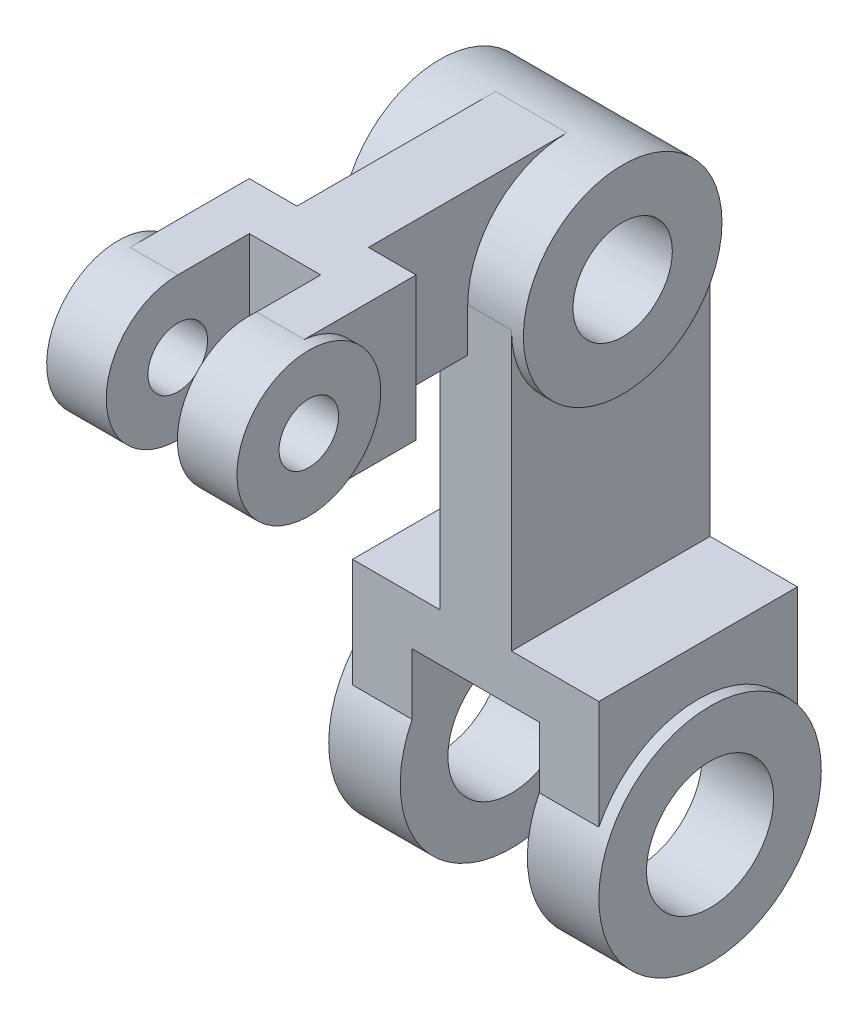
ISO-10303-21;
HEADER;
FILE_DESCRIPTION(('STEP AP214'),'2;1');
FILE_NAME('part.step','',(''),(''),'','','');
FILE_SCHEMA(('AUTOMOTIVE_DESIGN { 1 0 10303 214 1 1 1 1 }'));
ENDSEC;
DATA;
#1=APPLICATION_CONTEXT('core data for automotive mechanical design processes');
#2=APPLICATION_PROTOCOL_DEFINITION('international standard','automotive_design',2000,#1);
#3=PRODUCT_CONTEXT('',#1,'mechanical');
#4=PRODUCT('Part','Part','',(#3));
#5=PRODUCT_RELATED_PRODUCT_CATEGORY('part','',(#4));
#6=PRODUCT_DEFINITION_FORMATION('','',#4);
#7=PRODUCT_DEFINITION_CONTEXT('part definition',#1,'design');
#8=PRODUCT_DEFINITION('design','',#6,#7);
#9=PRODUCT_DEFINITION_SHAPE('','',#8);
#10=(LENGTH_UNIT() NAMED_UNIT(*) SI_UNIT(.MILLI.,.METRE.));
#11=(NAMED_UNIT(*) PLANE_ANGLE_UNIT() SI_UNIT($,.RADIAN.));
#12=(NAMED_UNIT(*) SI_UNIT($,.STERADIAN.) SOLID_ANGLE_UNIT());
#13=UNCERTAINTY_MEASURE_WITH_UNIT(LENGTH_MEASURE(1.E-05),#10,'distance_accuracy_value','');
#14=(GEOMETRIC_REPRESENTATION_CONTEXT(3) GLOBAL_UNCERTAINTY_ASSIGNED_CONTEXT((#13)) GLOBAL_UNIT_ASSIGNED_CONTEXT((#10,
#11,#12)) REPRESENTATION_CONTEXT('',''));
#15=CARTESIAN_POINT('',(0.,0.,0.));
#16=DIRECTION('',(0.,0.,1.));
#17=DIRECTION('',(1.,0.,0.));
#18=AXIS2_PLACEMENT_3D('',#15,#16,#17);
#19=CARTESIAN_POINT('',(-20.,71.,0.));
#20=DIRECTION('',(0.,-1.,0.));
#21=DIRECTION('',(0.,0.,-1.));
#22=AXIS2_PLACEMENT_3D('',#19,#20,#21);
#23=PLANE('',#22);
#24=DIRECTION('',(0.,0.,-1.));
#25=VECTOR('',#24,1.);
#26=CARTESIAN_POINT('',(9.99999999999999,71.,80.));
#27=LINE('',#26,#25);
#28=CARTESIAN_POINT('',(9.99999999999999,71.,78.13652597627));
#29=VERTEX_POINT('',#28);
#30=CARTESIAN_POINT('',(9.99999999999999,71.,50.));
#31=VERTEX_POINT('',#30);
#32=EDGE_CURVE('E226',#29,#31,#27,.T.);
#33=ORIENTED_EDGE('',*,*,#32,.F.);
#34=DIRECTION('',(-1.,0.,0.));
#35=VECTOR('',#34,1.);
#36=CARTESIAN_POINT('',(13.,71.,78.13652597627));
#37=LINE('',#36,#35);
#38=CARTESIAN_POINT('',(-2.00000000000001,71.,78.13652597627));
#39=VERTEX_POINT('',#38);
#40=EDGE_CURVE('E520',#29,#39,#37,.T.);
#41=ORIENTED_EDGE('',*,*,#40,.T.);
#42=DIRECTION('',(0.,0.,1.));
#43=VECTOR('',#42,1.);
#44=CARTESIAN_POINT('',(-2.00000000000001,71.,62.));
#45=LINE('',#44,#43);
#46=CARTESIAN_POINT('',(-2.00000000000001,71.,62.));
#47=VERTEX_POINT('',#46);
#48=EDGE_CURVE('E246',#47,#39,#45,.T.);
#49=ORIENTED_EDGE('',*,*,#48,.F.);
#50=DIRECTION('',(1.,0.,0.));
#51=VECTOR('',#50,1.);
#52=CARTESIAN_POINT('',(-2.00000000000001,71.,62.));
#53=LINE('',#52,#51);
#54=CARTESIAN_POINT('',(-20.,71.,62.));
#55=VERTEX_POINT('',#54);
#56=EDGE_CURVE('E244',#55,#47,#53,.T.);
#57=ORIENTED_EDGE('',*,*,#56,.F.);
#58=DIRECTION('',(0.,0.,1.));
#59=VECTOR('',#58,1.);
#60=CARTESIAN_POINT('',(-20.,71.,62.));
#61=LINE('',#60,#59);
#62=CARTESIAN_POINT('',(-20.,71.,80.));
#63=VERTEX_POINT('',#62);
#64=EDGE_CURVE('E234',#55,#63,#61,.T.);
#65=ORIENTED_EDGE('',*,*,#64,.T.);
#66=DIRECTION('',(1.,0.,0.));
#67=VECTOR('',#66,1.);
#68=CARTESIAN_POINT('',(-32.,71.,80.));
#69=LINE('',#68,#67);
#70=CARTESIAN_POINT('',(-32.,71.,80.));
#71=VERTEX_POINT('',#70);
#72=EDGE_CURVE('E218',#71,#63,#69,.T.);
#73=ORIENTED_EDGE('',*,*,#72,.F.);
#74=DIRECTION('',(0.,0.,-1.));
#75=VECTOR('',#74,1.);
#76=CARTESIAN_POINT('',(-32.,71.,80.));
#77=LINE('',#76,#75);
#78=CARTESIAN_POINT('',(-32.,71.,50.));
#79=VERTEX_POINT('',#78);
#80=EDGE_CURVE('E272',#71,#79,#77,.T.);
#81=ORIENTED_EDGE('',*,*,#80,.T.);
#82=DIRECTION('',(1.,0.,0.));
#83=VECTOR('',#82,1.);
#84=CARTESIAN_POINT('',(-32.,71.,50.));
#85=LINE('',#84,#83);
#86=CARTESIAN_POINT('',(-20.,71.,50.));
#87=VERTEX_POINT('',#86);
#88=EDGE_CURVE('E260',#79,#87,#85,.T.);
#89=ORIENTED_EDGE('',*,*,#88,.T.);
#90=DIRECTION('',(0.,0.,1.));
#91=VECTOR('',#90,1.);
#92=CARTESIAN_POINT('',(-20.,71.,0.));
#93=LINE('',#92,#91);
#94=CARTESIAN_POINT('',(-20.,71.,22.4499443206437));
#95=VERTEX_POINT('',#94);
#96=EDGE_CURVE('E293',#95,#87,#93,.T.);
#97=ORIENTED_EDGE('',*,*,#96,.F.);
#98=DIRECTION('',(1.,0.,0.));
#99=VECTOR('',#98,1.);
#100=CARTESIAN_POINT('',(-34.,71.,22.4499443206436));
#101=LINE('',#100,#99);
#102=CARTESIAN_POINT('',(-9.,71.,22.4499443206436));
#103=VERTEX_POINT('',#102);
#104=EDGE_CURVE('E287',#95,#103,#101,.T.);
#105=ORIENTED_EDGE('',*,*,#104,.T.);
#106=DIRECTION('',(0.,0.,-1.));
#107=VECTOR('',#106,1.);
#108=CARTESIAN_POINT('',(-9.,71.,-25.));
#109=LINE('',#108,#107);
#110=CARTESIAN_POINT('',(-9.,71.,25.));
#111=VERTEX_POINT('',#110);
#112=EDGE_CURVE('E294',#111,#103,#109,.T.);
#113=ORIENTED_EDGE('',*,*,#112,.F.);
#114=DIRECTION('',(-1.,0.,0.));
#115=VECTOR('',#114,1.);
#116=CARTESIAN_POINT('',(-31.,71.,25.));
#117=LINE('',#116,#115);
#118=CARTESIAN_POINT('',(-2.,71.,25.));
#119=VERTEX_POINT('',#118);
#120=EDGE_CURVE('E296',#119,#111,#117,.T.);
#121=ORIENTED_EDGE('',*,*,#120,.F.);
#122=DIRECTION('',(0.,0.,1.));
#123=VECTOR('',#122,1.);
#124=CARTESIAN_POINT('',(-2.,71.,0.));
#125=LINE('',#124,#123);
#126=CARTESIAN_POINT('',(-2.,71.,50.));
#127=VERTEX_POINT('',#126);
#128=EDGE_CURVE('E288',#119,#127,#125,.T.);
#129=ORIENTED_EDGE('',*,*,#128,.T.);
#130=EDGE_CURVE('E270',#127,#31,#85,.T.);
#131=ORIENTED_EDGE('',*,*,#130,.T.);
#132=EDGE_LOOP('',(#33,#41,#49,#57,#65,#73,#81,#89,#97,#105,#113,#121,#129,#131));
#133=FACE_BOUND('',#132,.T.);
#134=ADVANCED_FACE('F50',(#133),#23,.T.);
#135=CARTESIAN_POINT('',(-2.,107.,0.));
#136=DIRECTION('',(0.,1.,0.));
#137=DIRECTION('',(0.,0.,1.));
#138=AXIS2_PLACEMENT_3D('',#135,#136,#137);
#139=PLANE('',#138);
#140=DIRECTION('',(0.,0.,1.));
#141=VECTOR('',#140,1.);
#142=CARTESIAN_POINT('',(-2.00000000000002,107.,62.));
#143=LINE('',#142,#141);
#144=CARTESIAN_POINT('',(-2.00000000000002,107.,62.));
#145=VERTEX_POINT('',#144);
#146=CARTESIAN_POINT('',(-2.00000000000002,107.,78.13652597627));
#147=VERTEX_POINT('',#146);
#148=EDGE_CURVE('E249',#145,#147,#143,.T.);
#149=ORIENTED_EDGE('',*,*,#148,.T.);
#150=DIRECTION('',(-1.,0.,0.));
#151=VECTOR('',#150,1.);
#152=CARTESIAN_POINT('',(13.,107.,78.13652597627));
#153=LINE('',#152,#151);
#154=CARTESIAN_POINT('',(9.99999999999998,107.,78.13652597627));
#155=VERTEX_POINT('',#154);
#156=EDGE_CURVE('E511',#147,#155,#153,.F.);
#157=ORIENTED_EDGE('',*,*,#156,.T.);
#158=DIRECTION('',(0.,0.,-1.));
#159=VECTOR('',#158,1.);
#160=CARTESIAN_POINT('',(9.99999999999998,107.,80.));
#161=LINE('',#160,#159);
#162=CARTESIAN_POINT('',(9.99999999999998,107.,50.));
#163=VERTEX_POINT('',#162);
#164=EDGE_CURVE('E278',#155,#163,#161,.T.);
#165=ORIENTED_EDGE('',*,*,#164,.T.);
#166=DIRECTION('',(-1.,0.,0.));
#167=VECTOR('',#166,1.);
#168=CARTESIAN_POINT('',(-32.,107.,50.));
#169=LINE('',#168,#167);
#170=CARTESIAN_POINT('',(-2.00000000000001,107.,50.));
#171=VERTEX_POINT('',#170);
#172=EDGE_CURVE('E262',#163,#171,#169,.T.);
#173=ORIENTED_EDGE('',*,*,#172,.T.);
#174=DIRECTION('',(0.,0.,1.));
#175=VECTOR('',#174,1.);
#176=CARTESIAN_POINT('',(-2.,107.,0.));
#177=LINE('',#176,#175);
#178=CARTESIAN_POINT('',(-2.,107.,0.));
#179=VERTEX_POINT('',#178);
#180=EDGE_CURVE('E65',#179,#171,#177,.T.);
#181=ORIENTED_EDGE('',*,*,#180,.F.);
#182=DIRECTION('',(-1.,0.,0.));
#183=VECTOR('',#182,1.);
#184=CARTESIAN_POINT('',(-2.,107.,0.));
#185=LINE('',#184,#183);
#186=CARTESIAN_POINT('',(-20.,107.,0.));
#187=VERTEX_POINT('',#186);
#188=EDGE_CURVE('E285',#179,#187,#185,.T.);
#189=ORIENTED_EDGE('',*,*,#188,.T.);
#190=DIRECTION('',(0.,0.,1.));
#191=VECTOR('',#190,1.);
#192=CARTESIAN_POINT('',(-20.,107.,0.));
#193=LINE('',#192,#191);
#194=CARTESIAN_POINT('',(-20.,107.,50.));
#195=VERTEX_POINT('',#194);
#196=EDGE_CURVE('E286',#187,#195,#193,.T.);
#197=ORIENTED_EDGE('',*,*,#196,.T.);
#198=CARTESIAN_POINT('',(-32.,107.,50.));
#199=VERTEX_POINT('',#198);
#200=EDGE_CURVE('E264',#195,#199,#169,.T.);
#201=ORIENTED_EDGE('',*,*,#200,.T.);
#202=DIRECTION('',(0.,0.,-1.));
#203=VECTOR('',#202,1.);
#204=CARTESIAN_POINT('',(-32.,107.,80.));
#205=LINE('',#204,#203);
#206=CARTESIAN_POINT('',(-32.,107.,80.));
#207=VERTEX_POINT('',#206);
#208=EDGE_CURVE('E271',#207,#199,#205,.T.);
#209=ORIENTED_EDGE('',*,*,#208,.F.);
#210=DIRECTION('',(-1.,0.,0.));
#211=VECTOR('',#210,1.);
#212=CARTESIAN_POINT('',(-32.,107.,80.));
#213=LINE('',#212,#211);
#214=CARTESIAN_POINT('',(-20.,107.,80.));
#215=VERTEX_POINT('',#214);
#216=EDGE_CURVE('E230',#215,#207,#213,.T.);
#217=ORIENTED_EDGE('',*,*,#216,.F.);
#218=DIRECTION('',(0.,0.,1.));
#219=VECTOR('',#218,1.);
#220=CARTESIAN_POINT('',(-20.,107.,62.));
#221=LINE('',#220,#219);
#222=CARTESIAN_POINT('',(-20.,107.,62.));
#223=VERTEX_POINT('',#222);
#224=EDGE_CURVE('E240',#223,#215,#221,.T.);
#225=ORIENTED_EDGE('',*,*,#224,.F.);
#226=DIRECTION('',(-1.,0.,0.));
#227=VECTOR('',#226,1.);
#228=CARTESIAN_POINT('',(-20.,107.,62.));
#229=LINE('',#228,#227);
#230=EDGE_CURVE('E250',#145,#223,#229,.T.);
#231=ORIENTED_EDGE('',*,*,#230,.F.);
#232=EDGE_LOOP('',(#149,#157,#165,#173,#181,#189,#197,#201,#209,#217,#225,#231));
#233=FACE_BOUND('',#232,.T.);
#234=ADVANCED_FACE('F495',(#233),#139,.T.);
#235=CARTESIAN_POINT('',(-31.,12.,-25.));
#236=DIRECTION('',(0.,0.,1.));
#237=DIRECTION('',(1.,0.,0.));
#238=AXIS2_PLACEMENT_3D('',#235,#236,#237);
#239=PLANE('',#238);
#240=DIRECTION('',(1.,0.,0.));
#241=VECTOR('',#240,1.);
#242=CARTESIAN_POINT('',(-34.,-15.3904797870815,-25.));
#243=LINE('',#242,#241);
#244=CARTESIAN_POINT('',(-31.,-15.3904797870815,-25.));
#245=VERTEX_POINT('',#244);
#246=CARTESIAN_POINT('',(-16.,-15.3904797870815,-25.));
#247=VERTEX_POINT('',#246);
#248=EDGE_CURVE('E322',#245,#247,#243,.T.);
#249=ORIENTED_EDGE('',*,*,#248,.F.);
#250=DIRECTION('',(0.,-1.,0.));
#251=VECTOR('',#250,1.);
#252=CARTESIAN_POINT('',(-31.,12.,-25.));
#253=LINE('',#252,#251);
#254=CARTESIAN_POINT('',(-31.,12.,-25.));
#255=VERTEX_POINT('',#254);
#256=EDGE_CURVE('E54',#255,#245,#253,.T.);
#257=ORIENTED_EDGE('',*,*,#256,.F.);
#258=DIRECTION('',(-1.,0.,0.));
#259=VECTOR('',#258,1.);
#260=CARTESIAN_POINT('',(-31.,12.,-25.));
#261=LINE('',#260,#259);
#262=CARTESIAN_POINT('',(-9.,12.,-25.));
#263=VERTEX_POINT('',#262);
#264=EDGE_CURVE('E404',#263,#255,#261,.T.);
#265=ORIENTED_EDGE('',*,*,#264,.F.);
#266=DIRECTION('',(0.,-1.,0.));
#267=VECTOR('',#266,1.);
#268=CARTESIAN_POINT('',(-9.,82.,-25.));
#269=LINE('',#268,#267);
#270=CARTESIAN_POINT('',(-9.,82.,-25.));
#271=VERTEX_POINT('',#270);
#272=EDGE_CURVE('E400',#271,#263,#269,.T.);
#273=ORIENTED_EDGE('',*,*,#272,.F.);
#274=DIRECTION('',(-1.,0.,0.));
#275=VECTOR('',#274,1.);
#276=CARTESIAN_POINT('',(9.,82.,-25.));
#277=LINE('',#276,#275);
#278=CARTESIAN_POINT('',(9.,82.,-25.));
#279=VERTEX_POINT('',#278);
#280=EDGE_CURVE('E378',#279,#271,#277,.T.);
#281=ORIENTED_EDGE('',*,*,#280,.F.);
#282=DIRECTION('',(0.,-1.,0.));
#283=VECTOR('',#282,1.);
#284=CARTESIAN_POINT('',(9.,82.,-25.));
#285=LINE('',#284,#283);
#286=CARTESIAN_POINT('',(9.,12.,-25.));
#287=VERTEX_POINT('',#286);
#288=EDGE_CURVE('E383',#279,#287,#285,.T.);
#289=ORIENTED_EDGE('',*,*,#288,.T.);
#290=CARTESIAN_POINT('',(31.,12.,-25.));
#291=VERTEX_POINT('',#290);
#292=EDGE_CURVE('E408',#291,#287,#261,.T.);
#293=ORIENTED_EDGE('',*,*,#292,.F.);
#294=DIRECTION('',(0.,-1.,0.));
#295=VECTOR('',#294,1.);
#296=CARTESIAN_POINT('',(31.,12.,-25.));
#297=LINE('',#296,#295);
#298=CARTESIAN_POINT('',(31.,-15.3904797870815,-25.));
#299=VERTEX_POINT('',#298);
#300=EDGE_CURVE('E11',#291,#299,#297,.T.);
#301=ORIENTED_EDGE('',*,*,#300,.T.);
#302=DIRECTION('',(-1.,0.,0.));
#303=VECTOR('',#302,1.);
#304=CARTESIAN_POINT('',(34.,-15.3904797870815,-25.));
#305=LINE('',#304,#303);
#306=CARTESIAN_POINT('',(16.,-15.3904797870815,-25.));
#307=VERTEX_POINT('',#306);
#308=EDGE_CURVE('E351',#307,#299,#305,.F.);
#309=ORIENTED_EDGE('',*,*,#308,.F.);
#310=DIRECTION('',(0.,1.,0.));
#311=VECTOR('',#310,1.);
#312=CARTESIAN_POINT('',(16.,0.,-25.));
#313=LINE('',#312,#311);
#314=CARTESIAN_POINT('',(16.,0.,-25.));
#315=VERTEX_POINT('',#314);
#316=EDGE_CURVE('E358',#307,#315,#313,.T.);
#317=ORIENTED_EDGE('',*,*,#316,.T.);
#318=DIRECTION('',(-1.,0.,0.));
#319=VECTOR('',#318,1.);
#320=CARTESIAN_POINT('',(-31.,0.,-25.));
#321=LINE('',#320,#319);
#322=CARTESIAN_POINT('',(-16.,0.,-25.));
#323=VERTEX_POINT('',#322);
#324=EDGE_CURVE('E399',#315,#323,#321,.T.);
#325=ORIENTED_EDGE('',*,*,#324,.T.);
#326=DIRECTION('',(0.,-1.,0.));
#327=VECTOR('',#326,1.);
#328=CARTESIAN_POINT('',(-16.,0.,-25.));
#329=LINE('',#328,#327);
#330=EDGE_CURVE('E330',#323,#247,#329,.T.);
#331=ORIENTED_EDGE('',*,*,#330,.T.);
#332=EDGE_LOOP('',(#249,#257,#265,#273,#281,#289,#293,#301,#309,#317,#325,#331));
#333=FACE_BOUND('',#332,.T.);
#334=ADVANCED_FACE('F453',(#333),#239,.F.);
#335=CARTESIAN_POINT('',(-31.,12.,25.));
#336=DIRECTION('',(0.,0.,-1.));
#337=DIRECTION('',(-1.,0.,0.));
#338=AXIS2_PLACEMENT_3D('',#335,#336,#337);
#339=PLANE('',#338);
#340=DIRECTION('',(1.,0.,0.));
#341=VECTOR('',#340,1.);
#342=CARTESIAN_POINT('',(-9.,82.,25.));
#343=LINE('',#342,#341);
#344=CARTESIAN_POINT('',(-1.99999999999999,82.,25.));
#345=VERTEX_POINT('',#344);
#346=CARTESIAN_POINT('',(9.,82.,25.));
#347=VERTEX_POINT('',#346);
#348=EDGE_CURVE('E385',#345,#347,#343,.T.);
#349=ORIENTED_EDGE('',*,*,#348,.F.);
#350=DIRECTION('',(0.,-1.,0.));
#351=VECTOR('',#350,1.);
#352=CARTESIAN_POINT('',(-1.99999999999999,12.,25.));
#353=LINE('',#352,#351);
#354=EDGE_CURVE('E303',#345,#119,#353,.T.);
#355=ORIENTED_EDGE('',*,*,#354,.T.);
#356=ORIENTED_EDGE('',*,*,#120,.T.);
#357=DIRECTION('',(0.,-1.,0.));
#358=VECTOR('',#357,1.);
#359=CARTESIAN_POINT('',(-9.,82.,25.));
#360=LINE('',#359,#358);
#361=CARTESIAN_POINT('',(-9.,12.,25.));
#362=VERTEX_POINT('',#361);
#363=EDGE_CURVE('E391',#111,#362,#360,.T.);
#364=ORIENTED_EDGE('',*,*,#363,.T.);
#365=DIRECTION('',(1.,0.,0.));
#366=VECTOR('',#365,1.);
#367=CARTESIAN_POINT('',(-31.,12.,25.));
#368=LINE('',#367,#366);
#369=CARTESIAN_POINT('',(-31.,12.,25.));
#370=VERTEX_POINT('',#369);
#371=EDGE_CURVE('E413',#370,#362,#368,.T.);
#372=ORIENTED_EDGE('',*,*,#371,.F.);
#373=DIRECTION('',(0.,-1.,0.));
#374=VECTOR('',#373,1.);
#375=CARTESIAN_POINT('',(-31.,12.,25.));
#376=LINE('',#375,#374);
#377=CARTESIAN_POINT('',(-31.,-15.3904797870815,25.));
#378=VERTEX_POINT('',#377);
#379=EDGE_CURVE('E419',#370,#378,#376,.T.);
#380=ORIENTED_EDGE('',*,*,#379,.T.);
#381=DIRECTION('',(1.,0.,0.));
#382=VECTOR('',#381,1.);
#383=CARTESIAN_POINT('',(-34.,-15.3904797870815,25.));
#384=LINE('',#383,#382);
#385=CARTESIAN_POINT('',(-16.,-15.3904797870815,25.));
#386=VERTEX_POINT('',#385);
#387=EDGE_CURVE('E323',#386,#378,#384,.F.);
#388=ORIENTED_EDGE('',*,*,#387,.F.);
#389=DIRECTION('',(0.,1.,0.));
#390=VECTOR('',#389,1.);
#391=CARTESIAN_POINT('',(-16.,0.,25.));
#392=LINE('',#391,#390);
#393=CARTESIAN_POINT('',(-16.,0.,25.));
#394=VERTEX_POINT('',#393);
#395=EDGE_CURVE('E331',#386,#394,#392,.T.);
#396=ORIENTED_EDGE('',*,*,#395,.T.);
#397=DIRECTION('',(1.,0.,0.));
#398=VECTOR('',#397,1.);
#399=CARTESIAN_POINT('',(-31.,0.,25.));
#400=LINE('',#399,#398);
#401=CARTESIAN_POINT('',(16.,0.,25.));
#402=VERTEX_POINT('',#401);
#403=EDGE_CURVE('E403',#394,#402,#400,.T.);
#404=ORIENTED_EDGE('',*,*,#403,.T.);
#405=DIRECTION('',(0.,-1.,0.));
#406=VECTOR('',#405,1.);
#407=CARTESIAN_POINT('',(16.,-28.,25.));
#408=LINE('',#407,#406);
#409=CARTESIAN_POINT('',(16.,-15.3904797870815,25.));
#410=VERTEX_POINT('',#409);
#411=EDGE_CURVE('E353',#402,#410,#408,.T.);
#412=ORIENTED_EDGE('',*,*,#411,.T.);
#413=DIRECTION('',(-1.,0.,0.));
#414=VECTOR('',#413,1.);
#415=CARTESIAN_POINT('',(34.,-15.3904797870815,25.));
#416=LINE('',#415,#414);
#417=CARTESIAN_POINT('',(31.,-15.3904797870815,25.));
#418=VERTEX_POINT('',#417);
#419=EDGE_CURVE('E344',#418,#410,#416,.T.);
#420=ORIENTED_EDGE('',*,*,#419,.F.);
#421=DIRECTION('',(0.,-1.,0.));
#422=VECTOR('',#421,1.);
#423=CARTESIAN_POINT('',(31.,12.,25.));
#424=LINE('',#423,#422);
#425=CARTESIAN_POINT('',(31.,12.,25.));
#426=VERTEX_POINT('',#425);
#427=EDGE_CURVE('E415',#426,#418,#424,.T.);
#428=ORIENTED_EDGE('',*,*,#427,.F.);
#429=CARTESIAN_POINT('',(9.,12.,25.));
#430=VERTEX_POINT('',#429);
#431=EDGE_CURVE('E409',#430,#426,#368,.T.);
#432=ORIENTED_EDGE('',*,*,#431,.F.);
#433=DIRECTION('',(0.,-1.,0.));
#434=VECTOR('',#433,1.);
#435=CARTESIAN_POINT('',(9.,82.,25.));
#436=LINE('',#435,#434);
#437=EDGE_CURVE('E394',#347,#430,#436,.T.);
#438=ORIENTED_EDGE('',*,*,#437,.F.);
#439=EDGE_LOOP('',(#349,#355,#356,#364,#372,#380,#388,#396,#404,#412,#420,#428,#432,#438));
#440=FACE_BOUND('',#439,.T.);
#441=ADVANCED_FACE('F435',(#440),#339,.F.);
#442=CARTESIAN_POINT('',(0.,12.,0.));
#443=DIRECTION('',(0.,1.,0.));
#444=DIRECTION('',(0.,0.,1.));
#445=AXIS2_PLACEMENT_3D('',#442,#443,#444);
#446=PLANE('',#445);
#447=DIRECTION('',(0.,0.,-1.));
#448=VECTOR('',#447,1.);
#449=CARTESIAN_POINT('',(9.,12.,25.));
#450=LINE('',#449,#448);
#451=EDGE_CURVE('E384',#430,#287,#450,.T.);
#452=ORIENTED_EDGE('',*,*,#451,.F.);
#453=ORIENTED_EDGE('',*,*,#431,.T.);
#454=DIRECTION('',(0.,0.,-1.));
#455=VECTOR('',#454,1.);
#456=CARTESIAN_POINT('',(31.,12.,-25.));
#457=LINE('',#456,#455);
#458=EDGE_CURVE('E402',#426,#291,#457,.T.);
#459=ORIENTED_EDGE('',*,*,#458,.T.);
#460=ORIENTED_EDGE('',*,*,#292,.T.);
#461=EDGE_LOOP('',(#452,#453,#459,#460));
#462=FACE_BOUND('',#461,.T.);
#463=ADVANCED_FACE('F615',(#462),#446,.T.);
#464=CARTESIAN_POINT('',(31.,12.,-25.));
#465=DIRECTION('',(-1.,0.,0.));
#466=DIRECTION('',(0.,0.,1.));
#467=AXIS2_PLACEMENT_3D('',#464,#465,#466);
#468=PLANE('',#467);
#469=CARTESIAN_POINT('',(31.,-28.,0.));
#470=DIRECTION('',(-1.,0.,0.));
#471=DIRECTION('',(0.,0.,1.));
#472=AXIS2_PLACEMENT_3D('',#469,#470,#471);
#473=CIRCLE('',#472,28.);
#474=EDGE_CURVE('E347',#299,#418,#473,.F.);
#475=ORIENTED_EDGE('',*,*,#474,.F.);
#476=ORIENTED_EDGE('',*,*,#300,.F.);
#477=ORIENTED_EDGE('',*,*,#458,.F.);
#478=ORIENTED_EDGE('',*,*,#427,.T.);
#479=EDGE_LOOP('',(#475,#476,#477,#478));
#480=FACE_BOUND('',#479,.T.);
#481=ADVANCED_FACE('F47',(#480),#468,.F.);
#482=CARTESIAN_POINT('',(-31.,12.,-25.));
#483=DIRECTION('',(1.,0.,0.));
#484=DIRECTION('',(0.,0.,-1.));
#485=AXIS2_PLACEMENT_3D('',#482,#483,#484);
#486=PLANE('',#485);
#487=CARTESIAN_POINT('',(-31.,-28.,0.));
#488=DIRECTION('',(1.,0.,0.));
#489=DIRECTION('',(0.,0.,-1.));
#490=AXIS2_PLACEMENT_3D('',#487,#488,#489);
#491=CIRCLE('',#490,28.);
#492=EDGE_CURVE('E66',#378,#245,#491,.F.);
#493=ORIENTED_EDGE('',*,*,#492,.F.);
#494=ORIENTED_EDGE('',*,*,#379,.F.);
#495=DIRECTION('',(0.,0.,1.));
#496=VECTOR('',#495,1.);
#497=CARTESIAN_POINT('',(-31.,12.,-25.));
#498=LINE('',#497,#496);
#499=EDGE_CURVE('E406',#255,#370,#498,.T.);
#500=ORIENTED_EDGE('',*,*,#499,.F.);
#501=ORIENTED_EDGE('',*,*,#256,.T.);
#502=EDGE_LOOP('',(#493,#494,#500,#501));
#503=FACE_BOUND('',#502,.T.);
#504=ADVANCED_FACE('F421',(#503),#486,.F.);
#505=DIRECTION('',(0.,0.,1.));
#506=VECTOR('',#505,1.);
#507=CARTESIAN_POINT('',(-9.,12.,-25.));
#508=LINE('',#507,#506);
#509=EDGE_CURVE('E377',#263,#362,#508,.T.);
#510=ORIENTED_EDGE('',*,*,#509,.F.);
#511=ORIENTED_EDGE('',*,*,#264,.T.);
#512=ORIENTED_EDGE('',*,*,#499,.T.);
#513=ORIENTED_EDGE('',*,*,#371,.T.);
#514=EDGE_LOOP('',(#510,#511,#512,#513));
#515=FACE_BOUND('',#514,.T.);
#516=ADVANCED_FACE('F607',(#515),#446,.T.);
#517=CARTESIAN_POINT('',(0.,0.,0.));
#518=DIRECTION('',(0.,1.,0.));
#519=DIRECTION('',(0.,0.,1.));
#520=AXIS2_PLACEMENT_3D('',#517,#518,#519);
#521=PLANE('',#520);
#522=ORIENTED_EDGE('',*,*,#403,.F.);
#523=DIRECTION('',(0.,0.,-1.));
#524=VECTOR('',#523,1.);
#525=CARTESIAN_POINT('',(-16.,0.,-25.));
#526=LINE('',#525,#524);
#527=EDGE_CURVE('E329',#394,#323,#526,.T.);
#528=ORIENTED_EDGE('',*,*,#527,.T.);
#529=ORIENTED_EDGE('',*,*,#324,.F.);
#530=DIRECTION('',(0.,0.,1.));
#531=VECTOR('',#530,1.);
#532=CARTESIAN_POINT('',(16.,0.,25.));
#533=LINE('',#532,#531);
#534=EDGE_CURVE('E356',#315,#402,#533,.T.);
#535=ORIENTED_EDGE('',*,*,#534,.T.);
#536=EDGE_LOOP('',(#522,#528,#529,#535));
#537=FACE_BOUND('',#536,.T.);
#538=ADVANCED_FACE('F441',(#537),#521,.F.);
#539=CARTESIAN_POINT('',(-9.,82.,-25.));
#540=DIRECTION('',(1.,0.,0.));
#541=DIRECTION('',(0.,0.,-1.));
#542=AXIS2_PLACEMENT_3D('',#539,#540,#541);
#543=PLANE('',#542);
#544=ORIENTED_EDGE('',*,*,#363,.F.);
#545=ORIENTED_EDGE('',*,*,#112,.T.);
#546=CARTESIAN_POINT('',(-9.,82.,0.));
#547=DIRECTION('',(1.,0.,0.));
#548=DIRECTION('',(0.,0.,-1.));
#549=AXIS2_PLACEMENT_3D('',#546,#547,#548);
#550=CIRCLE('',#549,25.);
#551=EDGE_CURVE('E376',#103,#271,#550,.T.);
#552=ORIENTED_EDGE('',*,*,#551,.T.);
#553=ORIENTED_EDGE('',*,*,#272,.T.);
#554=ORIENTED_EDGE('',*,*,#509,.T.);
#555=EDGE_LOOP('',(#544,#545,#552,#553,#554));
#556=FACE_BOUND('',#555,.T.);
#557=ADVANCED_FACE('F480',(#556),#543,.F.);
#558=CARTESIAN_POINT('',(9.,82.,25.));
#559=DIRECTION('',(-1.,0.,0.));
#560=DIRECTION('',(0.,0.,1.));
#561=AXIS2_PLACEMENT_3D('',#558,#559,#560);
#562=PLANE('',#561);
#563=ORIENTED_EDGE('',*,*,#288,.F.);
#564=CARTESIAN_POINT('',(9.,82.,0.));
#565=DIRECTION('',(-1.,0.,0.));
#566=DIRECTION('',(0.,0.,1.));
#567=AXIS2_PLACEMENT_3D('',#564,#565,#566);
#568=CIRCLE('',#567,25.);
#569=EDGE_CURVE('E373',#279,#347,#568,.T.);
#570=ORIENTED_EDGE('',*,*,#569,.T.);
#571=ORIENTED_EDGE('',*,*,#437,.T.);
#572=ORIENTED_EDGE('',*,*,#451,.T.);
#573=EDGE_LOOP('',(#563,#570,#571,#572));
#574=FACE_BOUND('',#573,.T.);
#575=ADVANCED_FACE('F460',(#574),#562,.F.);
#576=CARTESIAN_POINT('',(-34.,82.,0.));
#577=DIRECTION('',(1.,0.,0.));
#578=DIRECTION('',(0.,0.,-1.));
#579=AXIS2_PLACEMENT_3D('',#576,#577,#578);
#580=CYLINDRICAL_SURFACE('',#579,25.);
#581=CARTESIAN_POINT('',(-1.99999999999999,82.,0.));
#582=DIRECTION('',(1.,0.,0.));
#583=DIRECTION('',(0.,1.,0.));
#584=AXIS2_PLACEMENT_3D('',#581,#582,#583);
#585=CIRCLE('',#584,25.);
#586=EDGE_CURVE('E301',#345,#179,#585,.F.);
#587=ORIENTED_EDGE('',*,*,#586,.F.);
#588=ORIENTED_EDGE('',*,*,#348,.T.);
#589=ORIENTED_EDGE('',*,*,#569,.F.);
#590=ORIENTED_EDGE('',*,*,#280,.T.);
#591=ORIENTED_EDGE('',*,*,#551,.F.);
#592=ORIENTED_EDGE('',*,*,#104,.F.);
#593=CARTESIAN_POINT('',(-20.,82.,0.));
#594=DIRECTION('',(-1.,0.,0.));
#595=DIRECTION('',(0.,-1.,0.));
#596=AXIS2_PLACEMENT_3D('',#593,#594,#595);
#597=CIRCLE('',#596,25.);
#598=EDGE_CURVE('E306',#187,#95,#597,.F.);
#599=ORIENTED_EDGE('',*,*,#598,.F.);
#600=ORIENTED_EDGE('',*,*,#188,.F.);
#601=EDGE_LOOP('',(#587,#588,#589,#590,#591,#592,#599,#600));
#602=FACE_BOUND('',#601,.T.);
#603=CARTESIAN_POINT('',(-34.,82.,0.));
#604=DIRECTION('',(1.,0.,0.));
#605=DIRECTION('',(0.,0.,-1.));
#606=AXIS2_PLACEMENT_3D('',#603,#604,#605);
#607=CIRCLE('',#606,25.);
#608=CARTESIAN_POINT('',(-34.,82.,-25.));
#609=VERTEX_POINT('',#608);
#610=EDGE_CURVE('E369',#609,#609,#607,.T.);
#611=ORIENTED_EDGE('',*,*,#610,.T.);
#612=EDGE_LOOP('',(#611));
#613=FACE_BOUND('',#612,.T.);
#614=CARTESIAN_POINT('',(12.,82.,0.));
#615=DIRECTION('',(1.,0.,0.));
#616=DIRECTION('',(0.,0.,-1.));
#617=AXIS2_PLACEMENT_3D('',#614,#615,#616);
#618=CIRCLE('',#617,25.);
#619=CARTESIAN_POINT('',(12.,82.,-25.));
#620=VERTEX_POINT('',#619);
#621=EDGE_CURVE('E364',#620,#620,#618,.T.);
#622=ORIENTED_EDGE('',*,*,#621,.F.);
#623=EDGE_LOOP('',(#622));
#624=FACE_BOUND('',#623,.T.);
#625=ADVANCED_FACE('F463',(#602,#613,#624),#580,.T.);
#626=CARTESIAN_POINT('',(-34.,82.,0.));
#627=DIRECTION('',(1.,0.,0.));
#628=DIRECTION('',(0.,0.,-1.));
#629=AXIS2_PLACEMENT_3D('',#626,#627,#628);
#630=PLANE('',#629);
#631=CARTESIAN_POINT('',(-34.,82.,0.));
#632=DIRECTION('',(1.,0.,0.));
#633=DIRECTION('',(0.,0.,-1.));
#634=AXIS2_PLACEMENT_3D('',#631,#632,#633);
#635=CIRCLE('',#634,12.5);
#636=CARTESIAN_POINT('',(-34.,82.,-12.5));
#637=VERTEX_POINT('',#636);
#638=EDGE_CURVE('E370',#637,#637,#635,.T.);
#639=ORIENTED_EDGE('',*,*,#638,.T.);
#640=EDGE_LOOP('',(#639));
#641=FACE_BOUND('',#640,.T.);
#642=ORIENTED_EDGE('',*,*,#610,.F.);
#643=EDGE_LOOP('',(#642));
#644=FACE_BOUND('',#643,.T.);
#645=ADVANCED_FACE('F600',(#641,#644),#630,.F.);
#646=CARTESIAN_POINT('',(-34.,82.,0.));
#647=DIRECTION('',(1.,0.,0.));
#648=DIRECTION('',(0.,0.,-1.));
#649=AXIS2_PLACEMENT_3D('',#646,#647,#648);
#650=CYLINDRICAL_SURFACE('',#649,12.5);
#651=ORIENTED_EDGE('',*,*,#638,.F.);
#652=EDGE_LOOP('',(#651));
#653=FACE_BOUND('',#652,.T.);
#654=CARTESIAN_POINT('',(12.,82.,0.));
#655=DIRECTION('',(1.,0.,0.));
#656=DIRECTION('',(0.,0.,-1.));
#657=AXIS2_PLACEMENT_3D('',#654,#655,#656);
#658=CIRCLE('',#657,12.5);
#659=CARTESIAN_POINT('',(12.,82.,-12.5));
#660=VERTEX_POINT('',#659);
#661=EDGE_CURVE('E363',#660,#660,#658,.T.);
#662=ORIENTED_EDGE('',*,*,#661,.T.);
#663=EDGE_LOOP('',(#662));
#664=FACE_BOUND('',#663,.T.);
#665=ADVANCED_FACE('F592',(#653,#664),#650,.F.);
#666=CARTESIAN_POINT('',(12.,82.,0.));
#667=DIRECTION('',(1.,0.,0.));
#668=DIRECTION('',(0.,0.,-1.));
#669=AXIS2_PLACEMENT_3D('',#666,#667,#668);
#670=PLANE('',#669);
#671=ORIENTED_EDGE('',*,*,#621,.T.);
#672=EDGE_LOOP('',(#671));
#673=FACE_BOUND('',#672,.T.);
#674=ORIENTED_EDGE('',*,*,#661,.F.);
#675=EDGE_LOOP('',(#674));
#676=FACE_BOUND('',#675,.T.);
#677=ADVANCED_FACE('F590',(#673,#676),#670,.T.);
#678=CARTESIAN_POINT('',(16.,0.,0.));
#679=DIRECTION('',(-1.,0.,0.));
#680=DIRECTION('',(0.,0.,1.));
#681=AXIS2_PLACEMENT_3D('',#678,#679,#680);
#682=PLANE('',#681);
#683=CARTESIAN_POINT('',(16.,-28.,0.));
#684=DIRECTION('',(1.,0.,0.));
#685=DIRECTION('',(0.,0.,-1.));
#686=AXIS2_PLACEMENT_3D('',#683,#684,#685);
#687=CIRCLE('',#686,16.);
#688=CARTESIAN_POINT('',(16.,-28.,-16.));
#689=VERTEX_POINT('',#688);
#690=EDGE_CURVE('E332',#689,#689,#687,.T.);
#691=ORIENTED_EDGE('',*,*,#690,.T.);
#692=EDGE_LOOP('',(#691));
#693=FACE_BOUND('',#692,.T.);
#694=ORIENTED_EDGE('',*,*,#316,.F.);
#695=CARTESIAN_POINT('',(16.,-28.,0.));
#696=DIRECTION('',(1.,0.,0.));
#697=DIRECTION('',(0.,0.,-1.));
#698=AXIS2_PLACEMENT_3D('',#695,#696,#697);
#699=CIRCLE('',#698,28.);
#700=EDGE_CURVE('E337',#410,#307,#699,.T.);
#701=ORIENTED_EDGE('',*,*,#700,.F.);
#702=ORIENTED_EDGE('',*,*,#411,.F.);
#703=ORIENTED_EDGE('',*,*,#534,.F.);
#704=EDGE_LOOP('',(#694,#701,#702,#703));
#705=FACE_BOUND('',#704,.T.);
#706=ADVANCED_FACE('F448',(#693,#705),#682,.T.);
#707=CARTESIAN_POINT('',(34.,-28.,0.));
#708=DIRECTION('',(-1.,0.,0.));
#709=DIRECTION('',(0.,0.,1.));
#710=AXIS2_PLACEMENT_3D('',#707,#708,#709);
#711=CYLINDRICAL_SURFACE('',#710,28.);
#712=CARTESIAN_POINT('',(34.,-28.,0.));
#713=DIRECTION('',(1.,0.,0.));
#714=DIRECTION('',(0.,0.,-1.));
#715=AXIS2_PLACEMENT_3D('',#712,#713,#714);
#716=CIRCLE('',#715,28.);
#717=CARTESIAN_POINT('',(34.,-28.,-28.));
#718=VERTEX_POINT('',#717);
#719=EDGE_CURVE('E345',#718,#718,#716,.T.);
#720=ORIENTED_EDGE('',*,*,#719,.F.);
#721=EDGE_LOOP('',(#720));
#722=FACE_BOUND('',#721,.T.);
#723=ORIENTED_EDGE('',*,*,#700,.T.);
#724=ORIENTED_EDGE('',*,*,#308,.T.);
#725=ORIENTED_EDGE('',*,*,#474,.T.);
#726=ORIENTED_EDGE('',*,*,#419,.T.);
#727=EDGE_LOOP('',(#723,#724,#725,#726));
#728=FACE_BOUND('',#727,.T.);
#729=ADVANCED_FACE('F449',(#722,#728),#711,.T.);
#730=CARTESIAN_POINT('',(34.,-28.,0.));
#731=DIRECTION('',(1.,0.,0.));
#732=DIRECTION('',(0.,0.,-1.));
#733=AXIS2_PLACEMENT_3D('',#730,#731,#732);
#734=PLANE('',#733);
#735=ORIENTED_EDGE('',*,*,#719,.T.);
#736=EDGE_LOOP('',(#735));
#737=FACE_BOUND('',#736,.T.);
#738=CARTESIAN_POINT('',(34.,-28.,0.));
#739=DIRECTION('',(1.,0.,0.));
#740=DIRECTION('',(0.,0.,-1.));
#741=AXIS2_PLACEMENT_3D('',#738,#739,#740);
#742=CIRCLE('',#741,16.);
#743=CARTESIAN_POINT('',(34.,-28.,-16.));
#744=VERTEX_POINT('',#743);
#745=EDGE_CURVE('E339',#744,#744,#742,.T.);
#746=ORIENTED_EDGE('',*,*,#745,.F.);
#747=EDGE_LOOP('',(#746));
#748=FACE_BOUND('',#747,.T.);
#749=ADVANCED_FACE('F576',(#737,#748),#734,.T.);
#750=CARTESIAN_POINT('',(34.,-28.,0.));
#751=DIRECTION('',(-1.,0.,0.));
#752=DIRECTION('',(0.,0.,1.));
#753=AXIS2_PLACEMENT_3D('',#750,#751,#752);
#754=CYLINDRICAL_SURFACE('',#753,16.);
#755=ORIENTED_EDGE('',*,*,#690,.F.);
#756=EDGE_LOOP('',(#755));
#757=FACE_BOUND('',#756,.T.);
#758=ORIENTED_EDGE('',*,*,#745,.T.);
#759=EDGE_LOOP('',(#758));
#760=FACE_BOUND('',#759,.T.);
#761=ADVANCED_FACE('F574',(#757,#760),#754,.F.);
#762=CARTESIAN_POINT('',(-16.,0.,0.));
#763=DIRECTION('',(1.,0.,0.));
#764=DIRECTION('',(0.,0.,-1.));
#765=AXIS2_PLACEMENT_3D('',#762,#763,#764);
#766=PLANE('',#765);
#767=CARTESIAN_POINT('',(-16.,-28.,0.));
#768=DIRECTION('',(-1.,0.,0.));
#769=DIRECTION('',(0.,0.,1.));
#770=AXIS2_PLACEMENT_3D('',#767,#768,#769);
#771=CIRCLE('',#770,16.);
#772=CARTESIAN_POINT('',(-16.,-28.,16.));
#773=VERTEX_POINT('',#772);
#774=EDGE_CURVE('E308',#773,#773,#771,.T.);
#775=ORIENTED_EDGE('',*,*,#774,.T.);
#776=EDGE_LOOP('',(#775));
#777=FACE_BOUND('',#776,.T.);
#778=ORIENTED_EDGE('',*,*,#395,.F.);
#779=CARTESIAN_POINT('',(-16.,-28.,0.));
#780=DIRECTION('',(-1.,0.,0.));
#781=DIRECTION('',(0.,0.,1.));
#782=AXIS2_PLACEMENT_3D('',#779,#780,#781);
#783=CIRCLE('',#782,28.);
#784=EDGE_CURVE('E311',#247,#386,#783,.T.);
#785=ORIENTED_EDGE('',*,*,#784,.F.);
#786=ORIENTED_EDGE('',*,*,#330,.F.);
#787=ORIENTED_EDGE('',*,*,#527,.F.);
#788=EDGE_LOOP('',(#778,#785,#786,#787));
#789=FACE_BOUND('',#788,.T.);
#790=ADVANCED_FACE('F436',(#777,#789),#766,.T.);
#791=CARTESIAN_POINT('',(-34.,-28.,0.));
#792=DIRECTION('',(1.,0.,0.));
#793=DIRECTION('',(0.,0.,-1.));
#794=AXIS2_PLACEMENT_3D('',#791,#792,#793);
#795=CYLINDRICAL_SURFACE('',#794,28.);
#796=CARTESIAN_POINT('',(-34.,-28.,0.));
#797=DIRECTION('',(-1.,0.,0.));
#798=DIRECTION('',(0.,0.,1.));
#799=AXIS2_PLACEMENT_3D('',#796,#797,#798);
#800=CIRCLE('',#799,28.);
#801=CARTESIAN_POINT('',(-34.,-28.,28.));
#802=VERTEX_POINT('',#801);
#803=EDGE_CURVE('E320',#802,#802,#800,.T.);
#804=ORIENTED_EDGE('',*,*,#803,.F.);
#805=EDGE_LOOP('',(#804));
#806=FACE_BOUND('',#805,.T.);
#807=ORIENTED_EDGE('',*,*,#492,.T.);
#808=ORIENTED_EDGE('',*,*,#248,.T.);
#809=ORIENTED_EDGE('',*,*,#784,.T.);
#810=ORIENTED_EDGE('',*,*,#387,.T.);
#811=EDGE_LOOP('',(#807,#808,#809,#810));
#812=FACE_BOUND('',#811,.T.);
#813=ADVANCED_FACE('F430',(#806,#812),#795,.T.);
#814=CARTESIAN_POINT('',(-34.,-28.,0.));
#815=DIRECTION('',(-1.,0.,0.));
#816=DIRECTION('',(0.,0.,1.));
#817=AXIS2_PLACEMENT_3D('',#814,#815,#816);
#818=PLANE('',#817);
#819=ORIENTED_EDGE('',*,*,#803,.T.);
#820=EDGE_LOOP('',(#819));
#821=FACE_BOUND('',#820,.T.);
#822=CARTESIAN_POINT('',(-34.,-28.,0.));
#823=DIRECTION('',(-1.,0.,0.));
#824=DIRECTION('',(0.,0.,1.));
#825=AXIS2_PLACEMENT_3D('',#822,#823,#824);
#826=CIRCLE('',#825,16.);
#827=CARTESIAN_POINT('',(-34.,-28.,16.));
#828=VERTEX_POINT('',#827);
#829=EDGE_CURVE('E313',#828,#828,#826,.T.);
#830=ORIENTED_EDGE('',*,*,#829,.F.);
#831=EDGE_LOOP('',(#830));
#832=FACE_BOUND('',#831,.T.);
#833=ADVANCED_FACE('F564',(#821,#832),#818,.T.);
#834=CARTESIAN_POINT('',(-34.,-28.,0.));
#835=DIRECTION('',(1.,0.,0.));
#836=DIRECTION('',(0.,0.,-1.));
#837=AXIS2_PLACEMENT_3D('',#834,#835,#836);
#838=CYLINDRICAL_SURFACE('',#837,16.);
#839=ORIENTED_EDGE('',*,*,#774,.F.);
#840=EDGE_LOOP('',(#839));
#841=FACE_BOUND('',#840,.T.);
#842=ORIENTED_EDGE('',*,*,#829,.T.);
#843=EDGE_LOOP('',(#842));
#844=FACE_BOUND('',#843,.T.);
#845=ADVANCED_FACE('F565',(#841,#844),#838,.F.);
#846=CARTESIAN_POINT('',(-2.,71.,0.));
#847=DIRECTION('',(1.,0.,0.));
#848=DIRECTION('',(0.,1.,0.));
#849=AXIS2_PLACEMENT_3D('',#846,#847,#848);
#850=PLANE('',#849);
#851=ORIENTED_EDGE('',*,*,#354,.F.);
#852=ORIENTED_EDGE('',*,*,#586,.T.);
#853=ORIENTED_EDGE('',*,*,#180,.T.);
#854=DIRECTION('',(0.,1.,0.));
#855=VECTOR('',#854,1.);
#856=CARTESIAN_POINT('',(-2.,71.,50.));
#857=LINE('',#856,#855);
#858=EDGE_CURVE('E283',#127,#171,#857,.T.);
#859=ORIENTED_EDGE('',*,*,#858,.F.);
#860=ORIENTED_EDGE('',*,*,#128,.F.);
#861=EDGE_LOOP('',(#851,#852,#853,#859,#860));
#862=FACE_BOUND('',#861,.T.);
#863=ADVANCED_FACE('F473',(#862),#850,.T.);
#864=CARTESIAN_POINT('',(-20.,107.,0.));
#865=DIRECTION('',(-1.,0.,0.));
#866=DIRECTION('',(0.,-1.,0.));
#867=AXIS2_PLACEMENT_3D('',#864,#865,#866);
#868=PLANE('',#867);
#869=ORIENTED_EDGE('',*,*,#196,.F.);
#870=ORIENTED_EDGE('',*,*,#598,.T.);
#871=ORIENTED_EDGE('',*,*,#96,.T.);
#872=DIRECTION('',(0.,-1.,0.));
#873=VECTOR('',#872,1.);
#874=CARTESIAN_POINT('',(-20.,107.,50.));
#875=LINE('',#874,#873);
#876=EDGE_CURVE('E276',#195,#87,#875,.T.);
#877=ORIENTED_EDGE('',*,*,#876,.F.);
#878=EDGE_LOOP('',(#869,#870,#871,#877));
#879=FACE_BOUND('',#878,.T.);
#880=ADVANCED_FACE('F482',(#879),#868,.T.);
#881=CARTESIAN_POINT('',(0.,0.,50.));
#882=DIRECTION('',(0.,0.,1.));
#883=DIRECTION('',(1.,0.,0.));
#884=AXIS2_PLACEMENT_3D('',#881,#882,#883);
#885=PLANE('',#884);
#886=ORIENTED_EDGE('',*,*,#200,.F.);
#887=ORIENTED_EDGE('',*,*,#876,.T.);
#888=ORIENTED_EDGE('',*,*,#88,.F.);
#889=DIRECTION('',(0.,-1.,0.));
#890=VECTOR('',#889,1.);
#891=CARTESIAN_POINT('',(-32.,107.,50.));
#892=LINE('',#891,#890);
#893=EDGE_CURVE('E261',#199,#79,#892,.T.);
#894=ORIENTED_EDGE('',*,*,#893,.F.);
#895=EDGE_LOOP('',(#886,#887,#888,#894));
#896=FACE_BOUND('',#895,.T.);
#897=ADVANCED_FACE('F490',(#896),#885,.F.);
#898=ORIENTED_EDGE('',*,*,#130,.F.);
#899=ORIENTED_EDGE('',*,*,#858,.T.);
#900=ORIENTED_EDGE('',*,*,#172,.F.);
#901=DIRECTION('',(0.,1.,0.));
#902=VECTOR('',#901,1.);
#903=CARTESIAN_POINT('',(9.99999999999998,107.,50.));
#904=LINE('',#903,#902);
#905=EDGE_CURVE('E257',#31,#163,#904,.T.);
#906=ORIENTED_EDGE('',*,*,#905,.F.);
#907=EDGE_LOOP('',(#898,#899,#900,#906));
#908=FACE_BOUND('',#907,.T.);
#909=ADVANCED_FACE('F537',(#908),#885,.F.);
#910=CARTESIAN_POINT('',(9.99999999999998,107.,80.));
#911=DIRECTION('',(-1.,0.,0.));
#912=DIRECTION('',(0.,-1.,0.));
#913=AXIS2_PLACEMENT_3D('',#910,#911,#912);
#914=PLANE('',#913);
#915=CARTESIAN_POINT('',(9.99999999999998,89.,80.));
#916=DIRECTION('',(-1.,0.,0.));
#917=DIRECTION('',(0.,-1.,0.));
#918=AXIS2_PLACEMENT_3D('',#915,#916,#917);
#919=CIRCLE('',#918,18.0962022379591);
#920=EDGE_CURVE('E515',#29,#155,#919,.F.);
#921=ORIENTED_EDGE('',*,*,#920,.F.);
#922=ORIENTED_EDGE('',*,*,#32,.T.);
#923=ORIENTED_EDGE('',*,*,#905,.T.);
#924=ORIENTED_EDGE('',*,*,#164,.F.);
#925=EDGE_LOOP('',(#921,#922,#923,#924));
#926=FACE_BOUND('',#925,.T.);
#927=ADVANCED_FACE('F538',(#926),#914,.F.);
#928=CARTESIAN_POINT('',(-32.,107.,80.));
#929=DIRECTION('',(1.,0.,0.));
#930=DIRECTION('',(0.,1.,0.));
#931=AXIS2_PLACEMENT_3D('',#928,#929,#930);
#932=PLANE('',#931);
#933=CARTESIAN_POINT('',(-32.,89.,80.));
#934=DIRECTION('',(1.,0.,0.));
#935=DIRECTION('',(0.,1.,0.));
#936=AXIS2_PLACEMENT_3D('',#933,#934,#935);
#937=CIRCLE('',#936,18.);
#938=EDGE_CURVE('E222',#207,#71,#937,.F.);
#939=ORIENTED_EDGE('',*,*,#938,.F.);
#940=ORIENTED_EDGE('',*,*,#208,.T.);
#941=ORIENTED_EDGE('',*,*,#893,.T.);
#942=ORIENTED_EDGE('',*,*,#80,.F.);
#943=EDGE_LOOP('',(#939,#940,#941,#942));
#944=FACE_BOUND('',#943,.T.);
#945=ADVANCED_FACE('F494',(#944),#932,.F.);
#946=CARTESIAN_POINT('',(-20.,71.,62.));
#947=DIRECTION('',(-1.,0.,0.));
#948=DIRECTION('',(0.,0.,1.));
#949=AXIS2_PLACEMENT_3D('',#946,#947,#948);
#950=PLANE('',#949);
#951=CARTESIAN_POINT('',(-20.,89.,80.));
#952=DIRECTION('',(-1.,0.,0.));
#953=DIRECTION('',(0.,-1.,0.));
#954=AXIS2_PLACEMENT_3D('',#951,#952,#953);
#955=CIRCLE('',#954,7.5);
#956=CARTESIAN_POINT('',(-20.,81.5,80.));
#957=VERTEX_POINT('',#956);
#958=EDGE_CURVE('E239',#957,#957,#955,.T.);
#959=ORIENTED_EDGE('',*,*,#958,.T.);
#960=EDGE_LOOP('',(#959));
#961=FACE_BOUND('',#960,.T.);
#962=ORIENTED_EDGE('',*,*,#224,.T.);
#963=CARTESIAN_POINT('',(-20.,89.,80.));
#964=DIRECTION('',(-1.,0.,0.));
#965=DIRECTION('',(0.,-1.,0.));
#966=AXIS2_PLACEMENT_3D('',#963,#964,#965);
#967=CIRCLE('',#966,18.);
#968=EDGE_CURVE('E216',#63,#215,#967,.T.);
#969=ORIENTED_EDGE('',*,*,#968,.F.);
#970=ORIENTED_EDGE('',*,*,#64,.F.);
#971=DIRECTION('',(0.,-1.,0.));
#972=VECTOR('',#971,1.);
#973=CARTESIAN_POINT('',(-20.,71.,62.));
#974=LINE('',#973,#972);
#975=EDGE_CURVE('E519',#223,#55,#974,.T.);
#976=ORIENTED_EDGE('',*,*,#975,.F.);
#977=EDGE_LOOP('',(#962,#969,#970,#976));
#978=FACE_BOUND('',#977,.T.);
#979=ADVANCED_FACE('F231',(#961,#978),#950,.F.);
#980=CARTESIAN_POINT('',(-2.00000000000002,107.,62.));
#981=DIRECTION('',(1.,0.,0.));
#982=DIRECTION('',(0.,1.,0.));
#983=AXIS2_PLACEMENT_3D('',#980,#981,#982);
#984=PLANE('',#983);
#985=CARTESIAN_POINT('',(-2.00000000000002,89.,80.));
#986=DIRECTION('',(1.,0.,0.));
#987=DIRECTION('',(0.,1.,0.));
#988=AXIS2_PLACEMENT_3D('',#985,#986,#987);
#989=CIRCLE('',#988,18.0962022379591);
#990=EDGE_CURVE('E497',#147,#39,#989,.T.);
#991=ORIENTED_EDGE('',*,*,#990,.F.);
#992=ORIENTED_EDGE('',*,*,#148,.F.);
#993=DIRECTION('',(0.,1.,0.));
#994=VECTOR('',#993,1.);
#995=CARTESIAN_POINT('',(-2.00000000000002,107.,62.));
#996=LINE('',#995,#994);
#997=EDGE_CURVE('E254',#47,#145,#996,.T.);
#998=ORIENTED_EDGE('',*,*,#997,.F.);
#999=ORIENTED_EDGE('',*,*,#48,.T.);
#1000=EDGE_LOOP('',(#991,#992,#998,#999));
#1001=FACE_BOUND('',#1000,.T.);
#1002=CARTESIAN_POINT('',(-2.00000000000002,89.,80.));
#1003=DIRECTION('',(1.,0.,0.));
#1004=DIRECTION('',(0.,1.,0.));
#1005=AXIS2_PLACEMENT_3D('',#1002,#1003,#1004);
#1006=CIRCLE('',#1005,7.5);
#1007=CARTESIAN_POINT('',(-2.00000000000002,96.5,80.));
#1008=VERTEX_POINT('',#1007);
#1009=EDGE_CURVE('E492',#1008,#1008,#1006,.T.);
#1010=ORIENTED_EDGE('',*,*,#1009,.T.);
#1011=EDGE_LOOP('',(#1010));
#1012=FACE_BOUND('',#1011,.T.);
#1013=ADVANCED_FACE('F528',(#1001,#1012),#984,.F.);
#1014=CARTESIAN_POINT('',(0.,0.,62.));
#1015=DIRECTION('',(0.,0.,-1.));
#1016=DIRECTION('',(-1.,0.,0.));
#1017=AXIS2_PLACEMENT_3D('',#1014,#1015,#1016);
#1018=PLANE('',#1017);
#1019=ORIENTED_EDGE('',*,*,#975,.T.);
#1020=ORIENTED_EDGE('',*,*,#56,.T.);
#1021=ORIENTED_EDGE('',*,*,#997,.T.);
#1022=ORIENTED_EDGE('',*,*,#230,.T.);
#1023=EDGE_LOOP('',(#1019,#1020,#1021,#1022));
#1024=FACE_BOUND('',#1023,.T.);
#1025=ADVANCED_FACE('F725',(#1024),#1018,.F.);
#1026=CARTESIAN_POINT('',(13.,89.,80.));
#1027=DIRECTION('',(1.,0.,0.));
#1028=DIRECTION('',(0.,1.,0.));
#1029=AXIS2_PLACEMENT_3D('',#1026,#1027,#1028);
#1030=PLANE('',#1029);
#1031=CARTESIAN_POINT('',(13.,89.,80.));
#1032=DIRECTION('',(1.,0.,0.));
#1033=DIRECTION('',(0.,1.,0.));
#1034=AXIS2_PLACEMENT_3D('',#1031,#1032,#1033);
#1035=CIRCLE('',#1034,18.0962022379591);
#1036=CARTESIAN_POINT('',(13.,107.096202237959,80.));
#1037=VERTEX_POINT('',#1036);
#1038=EDGE_CURVE('E508',#1037,#1037,#1035,.T.);
#1039=ORIENTED_EDGE('',*,*,#1038,.T.);
#1040=EDGE_LOOP('',(#1039));
#1041=FACE_BOUND('',#1040,.T.);
#1042=CARTESIAN_POINT('',(13.,89.,80.));
#1043=DIRECTION('',(1.,0.,0.));
#1044=DIRECTION('',(0.,1.,0.));
#1045=AXIS2_PLACEMENT_3D('',#1042,#1043,#1044);
#1046=CIRCLE('',#1045,7.5);
#1047=CARTESIAN_POINT('',(13.,96.5,80.));
#1048=VERTEX_POINT('',#1047);
#1049=EDGE_CURVE('E506',#1048,#1048,#1046,.T.);
#1050=ORIENTED_EDGE('',*,*,#1049,.F.);
#1051=EDGE_LOOP('',(#1050));
#1052=FACE_BOUND('',#1051,.T.);
#1053=ADVANCED_FACE('F729',(#1041,#1052),#1030,.T.);
#1054=CARTESIAN_POINT('',(13.,89.,80.));
#1055=DIRECTION('',(-1.,0.,0.));
#1056=DIRECTION('',(0.,-1.,0.));
#1057=AXIS2_PLACEMENT_3D('',#1054,#1055,#1056);
#1058=CYLINDRICAL_SURFACE('',#1057,18.0962022379591);
#1059=ORIENTED_EDGE('',*,*,#40,.F.);
#1060=ORIENTED_EDGE('',*,*,#920,.T.);
#1061=ORIENTED_EDGE('',*,*,#156,.F.);
#1062=ORIENTED_EDGE('',*,*,#990,.T.);
#1063=EDGE_LOOP('',(#1059,#1060,#1061,#1062));
#1064=FACE_BOUND('',#1063,.T.);
#1065=ORIENTED_EDGE('',*,*,#1038,.F.);
#1066=EDGE_LOOP('',(#1065));
#1067=FACE_BOUND('',#1066,.T.);
#1068=ADVANCED_FACE('F535',(#1064,#1067),#1058,.T.);
#1069=CARTESIAN_POINT('',(13.,89.,80.));
#1070=DIRECTION('',(-1.,0.,0.));
#1071=DIRECTION('',(0.,-1.,0.));
#1072=AXIS2_PLACEMENT_3D('',#1069,#1070,#1071);
#1073=CYLINDRICAL_SURFACE('',#1072,7.5);
#1074=ORIENTED_EDGE('',*,*,#1009,.F.);
#1075=EDGE_LOOP('',(#1074));
#1076=FACE_BOUND('',#1075,.T.);
#1077=ORIENTED_EDGE('',*,*,#1049,.T.);
#1078=EDGE_LOOP('',(#1077));
#1079=FACE_BOUND('',#1078,.T.);
#1080=ADVANCED_FACE('F743',(#1076,#1079),#1073,.F.);
#1081=CARTESIAN_POINT('',(-35.,89.,80.));
#1082=DIRECTION('',(-1.,0.,0.));
#1083=DIRECTION('',(0.,-1.,0.));
#1084=AXIS2_PLACEMENT_3D('',#1081,#1082,#1083);
#1085=PLANE('',#1084);
#1086=CARTESIAN_POINT('',(-35.,89.,80.));
#1087=DIRECTION('',(-1.,0.,0.));
#1088=DIRECTION('',(0.,-1.,0.));
#1089=AXIS2_PLACEMENT_3D('',#1086,#1087,#1088);
#1090=CIRCLE('',#1089,18.);
#1091=CARTESIAN_POINT('',(-35.,71.,80.));
#1092=VERTEX_POINT('',#1091);
#1093=EDGE_CURVE('E496',#1092,#1092,#1090,.T.);
#1094=ORIENTED_EDGE('',*,*,#1093,.T.);
#1095=EDGE_LOOP('',(#1094));
#1096=FACE_BOUND('',#1095,.T.);
#1097=CARTESIAN_POINT('',(-35.,89.,80.));
#1098=DIRECTION('',(-1.,0.,0.));
#1099=DIRECTION('',(0.,-1.,0.));
#1100=AXIS2_PLACEMENT_3D('',#1097,#1098,#1099);
#1101=CIRCLE('',#1100,7.5);
#1102=CARTESIAN_POINT('',(-35.,81.5,80.));
#1103=VERTEX_POINT('',#1102);
#1104=EDGE_CURVE('E237',#1103,#1103,#1101,.T.);
#1105=ORIENTED_EDGE('',*,*,#1104,.F.);
#1106=EDGE_LOOP('',(#1105));
#1107=FACE_BOUND('',#1106,.T.);
#1108=ADVANCED_FACE('F750',(#1096,#1107),#1085,.T.);
#1109=CARTESIAN_POINT('',(-35.,89.,80.));
#1110=DIRECTION('',(1.,0.,0.));
#1111=DIRECTION('',(0.,1.,0.));
#1112=AXIS2_PLACEMENT_3D('',#1109,#1110,#1111);
#1113=CYLINDRICAL_SURFACE('',#1112,18.);
#1114=ORIENTED_EDGE('',*,*,#72,.T.);
#1115=ORIENTED_EDGE('',*,*,#968,.T.);
#1116=ORIENTED_EDGE('',*,*,#216,.T.);
#1117=ORIENTED_EDGE('',*,*,#938,.T.);
#1118=EDGE_LOOP('',(#1114,#1115,#1116,#1117));
#1119=FACE_BOUND('',#1118,.T.);
#1120=ORIENTED_EDGE('',*,*,#1093,.F.);
#1121=EDGE_LOOP('',(#1120));
#1122=FACE_BOUND('',#1121,.T.);
#1123=ADVANCED_FACE('F217',(#1119,#1122),#1113,.T.);
#1124=CARTESIAN_POINT('',(-35.,89.,80.));
#1125=DIRECTION('',(1.,0.,0.));
#1126=DIRECTION('',(0.,1.,0.));
#1127=AXIS2_PLACEMENT_3D('',#1124,#1125,#1126);
#1128=CYLINDRICAL_SURFACE('',#1127,7.5);
#1129=ORIENTED_EDGE('',*,*,#958,.F.);
#1130=EDGE_LOOP('',(#1129));
#1131=FACE_BOUND('',#1130,.T.);
#1132=ORIENTED_EDGE('',*,*,#1104,.T.);
#1133=EDGE_LOOP('',(#1132));
#1134=FACE_BOUND('',#1133,.T.);
#1135=ADVANCED_FACE('F758',(#1131,#1134),#1128,.F.);
#1136=CLOSED_SHELL('',(#134,#234,#334,#441,#463,#481,#504,#516,#538,#557,#575,#625,#645,#665,
#677,#706,#729,#749,#761,#790,#813,#833,#845,#863,#880,#897,#909,#927,#945,#979,#1013,#1025,
#1053,#1068,#1080,#1108,#1123,#1135));
#1137=MANIFOLD_SOLID_BREP('B2',#1136);
#1138=ADVANCED_BREP_SHAPE_REPRESENTATION('',(#18,#1137),#14);
#1139=SHAPE_DEFINITION_REPRESENTATION(#9,#1138);
ENDSEC;
END-ISO-10303-21;
